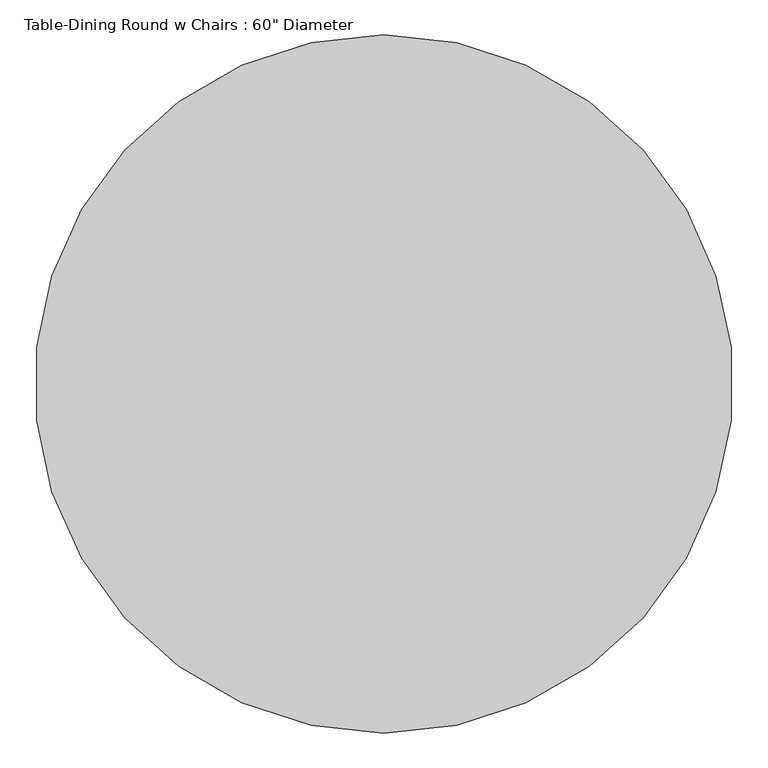
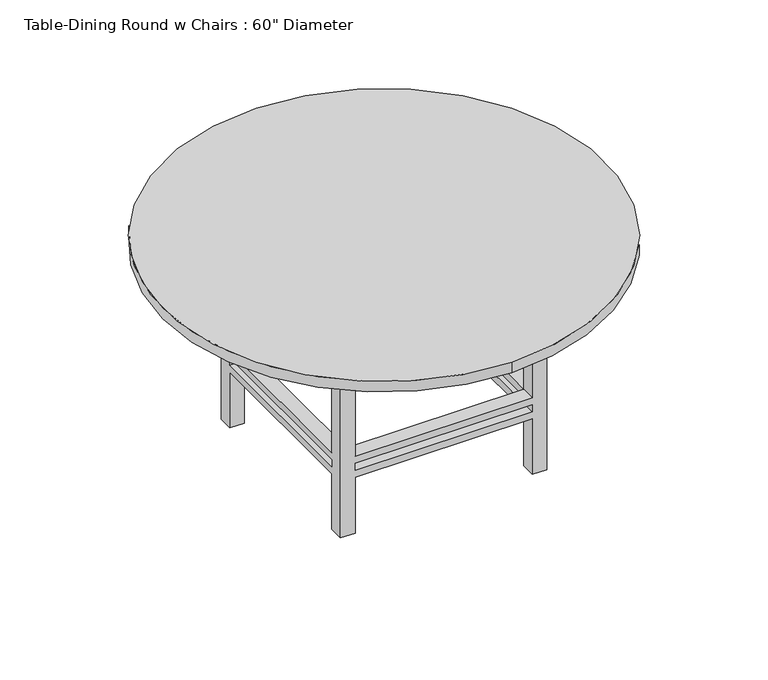
"""IFC4 building model written with IfcOpenShell, lengths in millimetres: furniture geometry."""

from ifc_helpers import new_model, si_unit, point, frame, frame_2d, origin, place, context, project, spatial, polyline, circle_curve, trimmed, segment, composite_curve, outline, extrude, faceted_brep, source, transform, mapped, element, save


def furniture_bbcc68ce(model_context):
    return source(origin(), model_context, "Body", "SolidModel", [
        faceted_brep([(408.4819672, 119.9213115, 279.4), (408.4819672, -489.6786885, 279.4), (459.2819672, -489.6786885, 279.4), (459.2819672, 119.9213115, 279.4), (-201.1180328, -489.6786885, 279.4), (-201.1180328, -540.4786885, 279.4), (408.4819672, -540.4786885, 279.4), (-201.1180328, 119.9213115, 279.4), (-251.9180328, 119.9213115, 279.4), (-251.9180328, -489.6786885, 279.4), (408.4819672, 170.7213115, 279.4), (-201.1180328, 170.7213115, 279.4), (408.4819672, 119.9213115, 254.0), (-201.1180328, 119.9213115, 254.0), (-201.1180328, 170.7213115, 254.0), (408.4819672, 170.7213115, 254.0), (-201.1180328, -489.6786885, 254.0), (-251.9180328, -489.6786885, 254.0), (-251.9180328, 119.9213115, 254.0), (408.4819672, -489.6786885, 254.0), (408.4819672, -540.4786885, 254.0), (-201.1180328, -540.4786885, 254.0), (459.2819672, 119.9213115, 254.0), (459.2819672, -489.6786885, 254.0), (-251.9180328, 170.7213115, 647.7), (-201.1180328, 170.7213115, 647.7), (408.4819672, 170.7213115, 647.7), (459.2819672, 170.7213115, 647.7), (459.2819672, 170.7213115, 0.0), (408.4819672, 170.7213115, 0.0), (408.4819672, 170.7213115, 203.2), (-201.1180328, 170.7213115, 203.2), (-201.1180328, 170.7213115, 0.0), (-251.9180328, 170.7213115, 0.0), (-201.1180328, 170.7213115, 228.6), (408.4819672, 170.7213115, 228.6), (-251.9180328, 119.9213115, 647.7), (-251.9180328, 119.9213115, 0.0), (-251.9180328, 119.9213115, 203.2), (-251.9180328, -489.6786885, 203.2), (-251.9180328, -489.6786885, 0.0), (-251.9180328, -540.4786885, 0.0), (-251.9180328, -540.4786885, 647.7), (-251.9180328, -489.6786885, 647.7), (-251.9180328, -489.6786885, 228.6), (-251.9180328, 119.9213115, 228.6), (459.2819672, -540.4786885, 647.7), (408.4819672, -540.4786885, 647.7), (-201.1180328, -540.4786885, 647.7), (-201.1180328, -540.4786885, 0.0), (-201.1180328, -540.4786885, 203.2), (408.4819672, -540.4786885, 203.2), (408.4819672, -540.4786885, 0.0), (459.2819672, -540.4786885, 0.0), (408.4819672, -540.4786885, 228.6), (-201.1180328, -540.4786885, 228.6), (459.2819672, 119.9213115, 647.7), (459.2819672, -489.6786885, 647.7), (459.2819672, -489.6786885, 0.0), (459.2819672, -489.6786885, 203.2), (459.2819672, 119.9213115, 203.2), (459.2819672, 119.9213115, 0.0), (459.2819672, 119.9213115, 228.6), (459.2819672, -489.6786885, 228.6), (-201.1180328, 119.9213115, 647.7), (408.4819672, -489.6786885, 647.7), (408.4819672, 119.9213115, 647.7), (-201.1180328, -489.6786885, 647.7), (408.4819672, 119.9213115, 0.0), (-201.1180328, -489.6786885, 0.0), (-201.1180328, 119.9213115, 0.0), (408.4819672, -489.6786885, 0.0), (-201.1180328, 119.9213115, 228.6), (-201.1180328, 119.9213115, 203.2), (408.4819672, 119.9213115, 228.6), (408.4819672, 119.9213115, 203.2), (408.4819672, -489.6786885, 228.6), (408.4819672, -489.6786885, 203.2), (-201.1180328, -489.6786885, 228.6), (-201.1180328, -489.6786885, 203.2)], [[[0, 1, 2, 3]], [[1, 4, 5, 6]], [[4, 7, 8, 9]], [[7, 0, 10, 11]], [[12, 13, 14, 15]], [[13, 16, 17, 18]], [[16, 19, 20, 21]], [[19, 12, 22, 23]], [[24, 25, 11, 10, 26, 27, 28, 29, 30, 31, 32, 33], [14, 34, 35, 15]], [[36, 24, 33, 37, 38, 39, 40, 41, 42, 43, 9, 8], [17, 44, 45, 18]], [[46, 47, 6, 5, 48, 42, 41, 49, 50, 51, 52, 53], [20, 54, 55, 21]], [[28, 27, 56, 3, 2, 57, 46, 53, 58, 59, 60, 61], [22, 62, 63, 23]], [[1, 0, 12, 19]], [[4, 1, 19, 16]], [[7, 4, 16, 13]], [[0, 7, 13, 12]], [[25, 24, 36, 64]], [[47, 46, 57, 65]], [[26, 66, 56, 27]], [[48, 67, 43, 42]], [[29, 28, 61, 68]], [[49, 41, 40, 69]], [[32, 70, 37, 33]], [[52, 71, 58, 53]], [[13, 18, 45, 72]], [[64, 36, 8, 7]], [[37, 70, 73, 38]], [[14, 13, 72, 34]], [[25, 64, 7, 11]], [[70, 32, 31, 73]], [[12, 15, 35, 74]], [[66, 26, 10, 0]], [[29, 68, 75, 30]], [[22, 12, 74, 62]], [[56, 66, 0, 3]], [[68, 61, 60, 75]], [[19, 23, 63, 76]], [[65, 57, 2, 1]], [[58, 71, 77, 59]], [[20, 19, 76, 54]], [[47, 65, 1, 6]], [[71, 52, 51, 77]], [[16, 21, 55, 78]], [[67, 48, 5, 4]], [[49, 69, 79, 50]], [[17, 16, 78, 44]], [[43, 67, 4, 9]], [[69, 40, 39, 79]], [[74, 76, 63, 62]], [[76, 78, 55, 54]], [[78, 72, 45, 44]], [[72, 74, 35, 34]], [[75, 73, 31, 30]], [[73, 79, 39, 38]], [[79, 77, 51, 50]], [[77, 75, 60, 59]], [[76, 74, 75, 77]], [[78, 76, 77, 79]], [[72, 78, 79, 73]], [[74, 72, 73, 75]]]),
        extrude(outline(polyline([(484.6819672, 196.1213115), (484.6819672, -565.8786885), (-277.3180328, -565.8786885), (-277.3180328, 196.1213115), (484.6819672, 196.1213115)]), holes=[polyline([(459.2819672, 170.7213115), (-251.9180328, 170.7213115), (-251.9180328, -540.4786885), (459.2819672, -540.4786885), (459.2819672, 170.7213115)])]), frame((0.0, 0.0, 647.7), z_axis=(0.0, 0.0, 1.0), x_axis=(1.0, 0.0, 0.0)), (0.0, 0.0, 1.0), 76.2),
        extrude(outline(composite_curve([segment(trimmed(circle_curve(frame_2d((103.6819672, -184.8786885)), 762.0), [point((103.6819672, -946.8786885))], [point((103.6819672, 577.1213115))], False, "CARTESIAN"), True, "CONTINUOUS"), segment(trimmed(circle_curve(frame_2d((103.6819672, -184.8786885)), 762.0), [point((103.6819672, 577.1213115))], [point((103.6819672, -946.8786885))], False, "CARTESIAN"), True, "CONTINUOUS")], self_intersect=False)), frame((0.0, 0.0, 723.9), z_axis=(0.0, 0.0, 1.0), x_axis=(1.0, 0.0, 0.0)), (0.0, 0.0, 1.0), 38.1),
    ])


if __name__ == "__main__":
    model = new_model("IFC4")
    model_context = context("Model", 3, world=origin())
    ifc_project = project(units=[si_unit("LENGTHUNIT", "METRE", prefix="MILLI")], contexts=[model_context])
    site = spatial("IfcSite", under=ifc_project)
    building = spatial("IfcBuilding", under=site)
    placement = place(None, origin())
    furniture_shape = furniture_bbcc68ce(model_context)
    element("IfcFurniture", 1, ObjectType="Table-Dining Round w Chairs : 60\" Diameter", at=placement, inside=building, context=model_context, shape_type="MappedRepresentation", body=[
        mapped(furniture_shape, transform((0.0, 0.0, 0.0), x_axis=(1.0, 0.0, 0.0), y_axis=(0.0, 1.0, 0.0), z_axis=(0.0, 0.0, 1.0))),
    ])
    save(model, "model.ifc")

# Revit data of these elements
# Type "Table-Dining Round w Chairs : 60\" Diameter"
#   Assembly Code = "E2020200"
#   Radius = 2' - 6"
#   Diameter = 5' - 0"
#   Height = 2' - 6"
#   Chairs = 6
#   Base Material = Pine
#   Top Material = Laminate, Linen, Matte
#   Default Elevation = 0
# Element 1 (IfcFurniture, "Table-Dining Round w Chairs : 60\" Diameter")
#   Materials on its faces: "Pine", "Laminate, Linen, Matte"
# Materials
#   "Pine": class "Wood", colour RGB 223 192 134, transparency 0, Description = "Pinus Echinata", Cost = 0
#   "Laminate, Linen, Matte": class "Plastic", colour RGB 249 239 230, transparency 0, Description = "Plastic Laminate - Linen, Matte", Cost = 0
